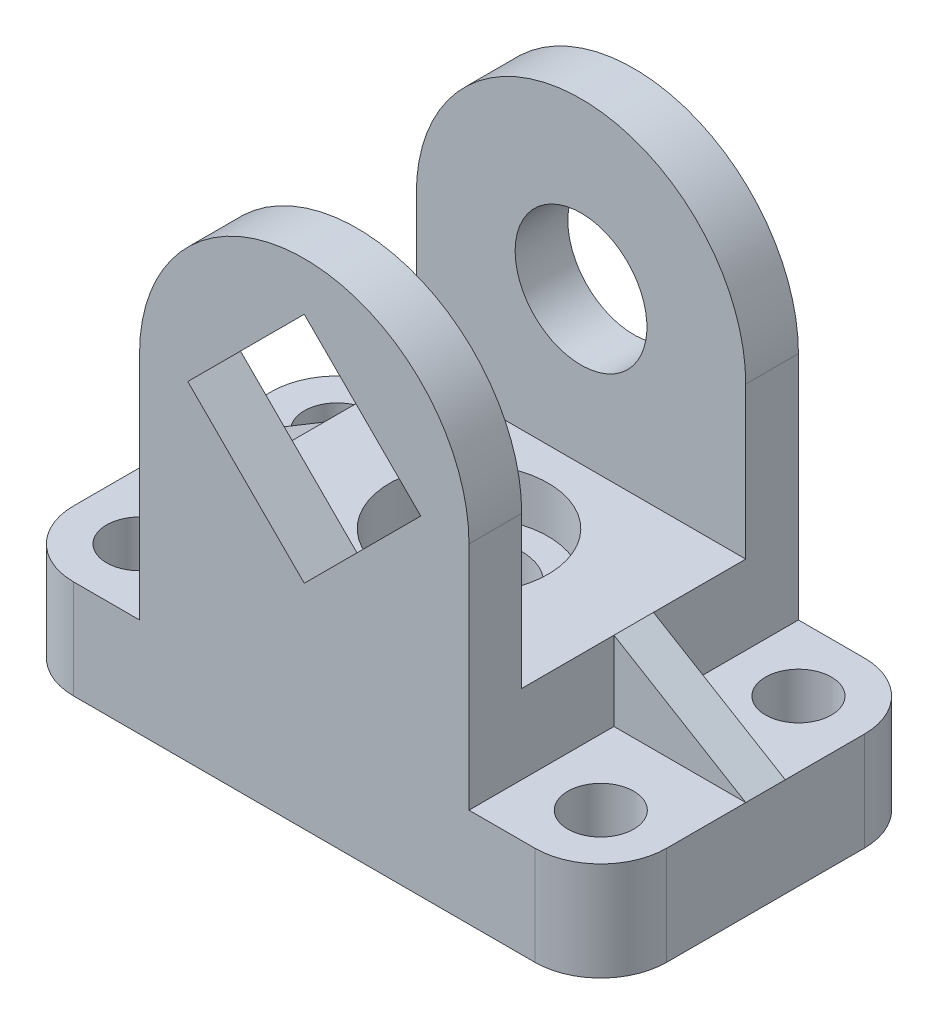
ISO-10303-21;
HEADER;
FILE_DESCRIPTION(('STEP AP214'),'2;1');
FILE_NAME('part.step','',(''),(''),'','','');
FILE_SCHEMA(('AUTOMOTIVE_DESIGN { 1 0 10303 214 1 1 1 1 }'));
ENDSEC;
DATA;
#1=APPLICATION_CONTEXT('core data for automotive mechanical design processes');
#2=APPLICATION_PROTOCOL_DEFINITION('international standard','automotive_design',2000,#1);
#3=PRODUCT_CONTEXT('',#1,'mechanical');
#4=PRODUCT('Part','Part','',(#3));
#5=PRODUCT_RELATED_PRODUCT_CATEGORY('part','',(#4));
#6=PRODUCT_DEFINITION_FORMATION('','',#4);
#7=PRODUCT_DEFINITION_CONTEXT('part definition',#1,'design');
#8=PRODUCT_DEFINITION('design','',#6,#7);
#9=PRODUCT_DEFINITION_SHAPE('','',#8);
#10=(LENGTH_UNIT() NAMED_UNIT(*) SI_UNIT(.MILLI.,.METRE.));
#11=(NAMED_UNIT(*) PLANE_ANGLE_UNIT() SI_UNIT($,.RADIAN.));
#12=(NAMED_UNIT(*) SI_UNIT($,.STERADIAN.) SOLID_ANGLE_UNIT());
#13=UNCERTAINTY_MEASURE_WITH_UNIT(LENGTH_MEASURE(1.E-05),#10,'distance_accuracy_value','');
#14=(GEOMETRIC_REPRESENTATION_CONTEXT(3) GLOBAL_UNCERTAINTY_ASSIGNED_CONTEXT((#13)) GLOBAL_UNIT_ASSIGNED_CONTEXT((#10,
#11,#12)) REPRESENTATION_CONTEXT('',''));
#15=CARTESIAN_POINT('',(0.,0.,0.));
#16=DIRECTION('',(0.,0.,1.));
#17=DIRECTION('',(1.,0.,0.));
#18=AXIS2_PLACEMENT_3D('',#15,#16,#17);
#19=CARTESIAN_POINT('',(-35.,15.,15.));
#20=DIRECTION('',(0.,-1.,0.));
#21=DIRECTION('',(0.,0.,-1.));
#22=AXIS2_PLACEMENT_3D('',#19,#20,#21);
#23=PLANE('',#22);
#24=CARTESIAN_POINT('',(-35.,15.,-15.));
#25=DIRECTION('',(0.,1.,0.));
#26=DIRECTION('',(0.,0.,1.));
#27=AXIS2_PLACEMENT_3D('',#24,#25,#26);
#28=CIRCLE('',#27,5.);
#29=CARTESIAN_POINT('',(-35.,15.,-10.));
#30=VERTEX_POINT('',#29);
#31=EDGE_CURVE('E380',#30,#30,#28,.T.);
#32=ORIENTED_EDGE('',*,*,#31,.F.);
#33=EDGE_LOOP('',(#32));
#34=FACE_BOUND('',#33,.T.);
#35=DIRECTION('',(-1.,0.,0.));
#36=VECTOR('',#35,1.);
#37=CARTESIAN_POINT('',(-35.,15.,-3.));
#38=LINE('',#37,#36);
#39=CARTESIAN_POINT('',(-25.,15.,-3.));
#40=VERTEX_POINT('',#39);
#41=CARTESIAN_POINT('',(-45.,15.,-3.));
#42=VERTEX_POINT('',#41);
#43=EDGE_CURVE('E230',#40,#42,#38,.T.);
#44=ORIENTED_EDGE('',*,*,#43,.F.);
#45=DIRECTION('',(0.,0.,1.));
#46=VECTOR('',#45,1.);
#47=CARTESIAN_POINT('',(-25.,15.,17.));
#48=LINE('',#47,#46);
#49=CARTESIAN_POINT('',(-25.,15.,-25.));
#50=VERTEX_POINT('',#49);
#51=EDGE_CURVE('E234',#50,#40,#48,.T.);
#52=ORIENTED_EDGE('',*,*,#51,.F.);
#53=DIRECTION('',(-1.,0.,0.));
#54=VECTOR('',#53,1.);
#55=CARTESIAN_POINT('',(-35.,15.,-25.));
#56=LINE('',#55,#54);
#57=CARTESIAN_POINT('',(-35.,15.,-25.));
#58=VERTEX_POINT('',#57);
#59=EDGE_CURVE('E396',#50,#58,#56,.T.);
#60=ORIENTED_EDGE('',*,*,#59,.T.);
#61=CARTESIAN_POINT('',(-35.,15.,-15.));
#62=DIRECTION('',(0.,1.,0.));
#63=DIRECTION('',(0.,0.,-1.));
#64=AXIS2_PLACEMENT_3D('',#61,#62,#63);
#65=CIRCLE('',#64,10.);
#66=CARTESIAN_POINT('',(-45.,15.,-15.));
#67=VERTEX_POINT('',#66);
#68=EDGE_CURVE('E399',#58,#67,#65,.T.);
#69=ORIENTED_EDGE('',*,*,#68,.T.);
#70=DIRECTION('',(0.,0.,1.));
#71=VECTOR('',#70,1.);
#72=CARTESIAN_POINT('',(-45.,15.,15.));
#73=LINE('',#72,#71);
#74=EDGE_CURVE('E401',#67,#42,#73,.T.);
#75=ORIENTED_EDGE('',*,*,#74,.T.);
#76=EDGE_LOOP('',(#44,#52,#60,#69,#75));
#77=FACE_BOUND('',#76,.T.);
#78=ADVANCED_FACE('F39',(#34,#77),#23,.F.);
#79=CARTESIAN_POINT('',(-25.,15.,17.));
#80=DIRECTION('',(-1.,0.,0.));
#81=DIRECTION('',(0.,0.,1.));
#82=AXIS2_PLACEMENT_3D('',#79,#80,#81);
#83=PLANE('',#82);
#84=ORIENTED_EDGE('',*,*,#51,.T.);
#85=DIRECTION('',(0.,1.,0.));
#86=VECTOR('',#85,1.);
#87=CARTESIAN_POINT('',(-25.,15.,-3.));
#88=LINE('',#87,#86);
#89=CARTESIAN_POINT('',(-25.,27.,-3.));
#90=VERTEX_POINT('',#89);
#91=EDGE_CURVE('E223',#40,#90,#88,.T.);
#92=ORIENTED_EDGE('',*,*,#91,.T.);
#93=DIRECTION('',(0.,0.,1.));
#94=VECTOR('',#93,1.);
#95=CARTESIAN_POINT('',(-25.,27.,-17.));
#96=LINE('',#95,#94);
#97=CARTESIAN_POINT('',(-25.,27.,-17.));
#98=VERTEX_POINT('',#97);
#99=EDGE_CURVE('E218',#98,#90,#96,.T.);
#100=ORIENTED_EDGE('',*,*,#99,.F.);
#101=DIRECTION('',(0.,-1.,0.));
#102=VECTOR('',#101,1.);
#103=CARTESIAN_POINT('',(-25.,15.,-17.));
#104=LINE('',#103,#102);
#105=CARTESIAN_POINT('',(-25.,50.,-17.));
#106=VERTEX_POINT('',#105);
#107=EDGE_CURVE('E497',#106,#98,#104,.T.);
#108=ORIENTED_EDGE('',*,*,#107,.F.);
#109=DIRECTION('',(0.,0.,-1.));
#110=VECTOR('',#109,1.);
#111=CARTESIAN_POINT('',(-25.,50.,-17.));
#112=LINE('',#111,#110);
#113=CARTESIAN_POINT('',(-25.,50.,-25.));
#114=VERTEX_POINT('',#113);
#115=EDGE_CURVE('E477',#106,#114,#112,.T.);
#116=ORIENTED_EDGE('',*,*,#115,.T.);
#117=DIRECTION('',(0.,-1.,0.));
#118=VECTOR('',#117,1.);
#119=CARTESIAN_POINT('',(-25.,15.,-25.));
#120=LINE('',#119,#118);
#121=EDGE_CURVE('E496',#114,#50,#120,.T.);
#122=ORIENTED_EDGE('',*,*,#121,.T.);
#123=EDGE_LOOP('',(#84,#92,#100,#108,#116,#122));
#124=FACE_BOUND('',#123,.T.);
#125=ADVANCED_FACE('F235',(#124),#83,.T.);
#126=CARTESIAN_POINT('',(35.,15.,-15.));
#127=DIRECTION('',(0.,1.,0.));
#128=DIRECTION('',(0.,0.,1.));
#129=AXIS2_PLACEMENT_3D('',#126,#127,#128);
#130=CIRCLE('',#129,5.);
#131=CARTESIAN_POINT('',(35.,15.,-10.));
#132=VERTEX_POINT('',#131);
#133=EDGE_CURVE('E371',#132,#132,#130,.T.);
#134=ORIENTED_EDGE('',*,*,#133,.F.);
#135=EDGE_LOOP('',(#134));
#136=FACE_BOUND('',#135,.T.);
#137=DIRECTION('',(-1.,0.,0.));
#138=VECTOR('',#137,1.);
#139=CARTESIAN_POINT('',(-35.,15.,-3.));
#140=LINE('',#139,#138);
#141=CARTESIAN_POINT('',(45.,15.,-3.));
#142=VERTEX_POINT('',#141);
#143=CARTESIAN_POINT('',(25.,15.,-3.));
#144=VERTEX_POINT('',#143);
#145=EDGE_CURVE('E256',#142,#144,#140,.T.);
#146=ORIENTED_EDGE('',*,*,#145,.F.);
#147=DIRECTION('',(0.,0.,-1.));
#148=VECTOR('',#147,1.);
#149=CARTESIAN_POINT('',(45.,15.,15.));
#150=LINE('',#149,#148);
#151=CARTESIAN_POINT('',(45.,15.,-15.));
#152=VERTEX_POINT('',#151);
#153=EDGE_CURVE('E388',#142,#152,#150,.T.);
#154=ORIENTED_EDGE('',*,*,#153,.T.);
#155=CARTESIAN_POINT('',(35.,15.,-15.));
#156=DIRECTION('',(0.,1.,0.));
#157=DIRECTION('',(0.,0.,-1.));
#158=AXIS2_PLACEMENT_3D('',#155,#156,#157);
#159=CIRCLE('',#158,10.);
#160=CARTESIAN_POINT('',(35.,15.,-25.));
#161=VERTEX_POINT('',#160);
#162=EDGE_CURVE('E392',#152,#161,#159,.T.);
#163=ORIENTED_EDGE('',*,*,#162,.T.);
#164=CARTESIAN_POINT('',(25.,15.,-25.));
#165=VERTEX_POINT('',#164);
#166=EDGE_CURVE('E400',#161,#165,#56,.T.);
#167=ORIENTED_EDGE('',*,*,#166,.T.);
#168=DIRECTION('',(0.,0.,1.));
#169=VECTOR('',#168,1.);
#170=CARTESIAN_POINT('',(25.,15.,17.));
#171=LINE('',#170,#169);
#172=EDGE_CURVE('E360',#165,#144,#171,.T.);
#173=ORIENTED_EDGE('',*,*,#172,.T.);
#174=EDGE_LOOP('',(#146,#154,#163,#167,#173));
#175=FACE_BOUND('',#174,.T.);
#176=ADVANCED_FACE('F304',(#136,#175),#23,.F.);
#177=CARTESIAN_POINT('',(25.,50.,17.));
#178=DIRECTION('',(1.,0.,0.));
#179=DIRECTION('',(0.,1.,0.));
#180=AXIS2_PLACEMENT_3D('',#177,#178,#179);
#181=PLANE('',#180);
#182=DIRECTION('',(0.,0.,-1.));
#183=VECTOR('',#182,1.);
#184=CARTESIAN_POINT('',(25.,27.,-17.));
#185=LINE('',#184,#183);
#186=CARTESIAN_POINT('',(25.,27.,-3.));
#187=VERTEX_POINT('',#186);
#188=CARTESIAN_POINT('',(25.,27.,-17.));
#189=VERTEX_POINT('',#188);
#190=EDGE_CURVE('E242',#187,#189,#185,.T.);
#191=ORIENTED_EDGE('',*,*,#190,.F.);
#192=DIRECTION('',(0.,-1.,0.));
#193=VECTOR('',#192,1.);
#194=CARTESIAN_POINT('',(25.,50.,-3.));
#195=LINE('',#194,#193);
#196=EDGE_CURVE('E257',#187,#144,#195,.T.);
#197=ORIENTED_EDGE('',*,*,#196,.T.);
#198=ORIENTED_EDGE('',*,*,#172,.F.);
#199=DIRECTION('',(0.,1.,0.));
#200=VECTOR('',#199,1.);
#201=CARTESIAN_POINT('',(25.,50.,-25.));
#202=LINE('',#201,#200);
#203=CARTESIAN_POINT('',(25.,50.,-25.));
#204=VERTEX_POINT('',#203);
#205=EDGE_CURVE('E493',#165,#204,#202,.T.);
#206=ORIENTED_EDGE('',*,*,#205,.T.);
#207=DIRECTION('',(0.,0.,-1.));
#208=VECTOR('',#207,1.);
#209=CARTESIAN_POINT('',(25.,50.,-17.));
#210=LINE('',#209,#208);
#211=CARTESIAN_POINT('',(25.,50.,-17.));
#212=VERTEX_POINT('',#211);
#213=EDGE_CURVE('E480',#212,#204,#210,.T.);
#214=ORIENTED_EDGE('',*,*,#213,.F.);
#215=DIRECTION('',(0.,1.,0.));
#216=VECTOR('',#215,1.);
#217=CARTESIAN_POINT('',(25.,50.,-17.));
#218=LINE('',#217,#216);
#219=EDGE_CURVE('E495',#189,#212,#218,.T.);
#220=ORIENTED_EDGE('',*,*,#219,.F.);
#221=EDGE_LOOP('',(#191,#197,#198,#206,#214,#220));
#222=FACE_BOUND('',#221,.T.);
#223=ADVANCED_FACE('F318',(#222),#181,.T.);
#224=CARTESIAN_POINT('',(-35.,15.,15.));
#225=DIRECTION('',(0.,1.,0.));
#226=DIRECTION('',(0.,0.,1.));
#227=AXIS2_PLACEMENT_3D('',#224,#225,#226);
#228=CIRCLE('',#227,5.);
#229=CARTESIAN_POINT('',(-35.,15.,20.));
#230=VERTEX_POINT('',#229);
#231=EDGE_CURVE('E338',#230,#230,#228,.T.);
#232=ORIENTED_EDGE('',*,*,#231,.F.);
#233=EDGE_LOOP('',(#232));
#234=FACE_BOUND('',#233,.T.);
#235=CARTESIAN_POINT('',(-25.,15.,3.));
#236=VERTEX_POINT('',#235);
#237=CARTESIAN_POINT('',(-25.,15.,25.));
#238=VERTEX_POINT('',#237);
#239=EDGE_CURVE('E337',#236,#238,#48,.T.);
#240=ORIENTED_EDGE('',*,*,#239,.F.);
#241=DIRECTION('',(-1.,0.,0.));
#242=VECTOR('',#241,1.);
#243=CARTESIAN_POINT('',(-35.,15.,3.));
#244=LINE('',#243,#242);
#245=CARTESIAN_POINT('',(-45.,15.,3.));
#246=VERTEX_POINT('',#245);
#247=EDGE_CURVE('E268',#236,#246,#244,.T.);
#248=ORIENTED_EDGE('',*,*,#247,.T.);
#249=CARTESIAN_POINT('',(-45.,15.,15.));
#250=VERTEX_POINT('',#249);
#251=EDGE_CURVE('E405',#246,#250,#73,.T.);
#252=ORIENTED_EDGE('',*,*,#251,.T.);
#253=CARTESIAN_POINT('',(-35.,15.,15.));
#254=DIRECTION('',(0.,1.,0.));
#255=DIRECTION('',(0.,0.,-1.));
#256=AXIS2_PLACEMENT_3D('',#253,#254,#255);
#257=CIRCLE('',#256,10.);
#258=CARTESIAN_POINT('',(-35.,15.,25.));
#259=VERTEX_POINT('',#258);
#260=EDGE_CURVE('E382',#250,#259,#257,.T.);
#261=ORIENTED_EDGE('',*,*,#260,.T.);
#262=DIRECTION('',(1.,0.,0.));
#263=VECTOR('',#262,1.);
#264=CARTESIAN_POINT('',(-35.,15.,25.));
#265=LINE('',#264,#263);
#266=EDGE_CURVE('E345',#259,#238,#265,.T.);
#267=ORIENTED_EDGE('',*,*,#266,.T.);
#268=EDGE_LOOP('',(#240,#248,#252,#261,#267));
#269=FACE_BOUND('',#268,.T.);
#270=ADVANCED_FACE('F308',(#234,#269),#23,.F.);
#271=CARTESIAN_POINT('',(35.,15.,15.));
#272=DIRECTION('',(0.,1.,0.));
#273=DIRECTION('',(0.,0.,1.));
#274=AXIS2_PLACEMENT_3D('',#271,#272,#273);
#275=CIRCLE('',#274,5.);
#276=CARTESIAN_POINT('',(35.,15.,20.));
#277=VERTEX_POINT('',#276);
#278=EDGE_CURVE('E363',#277,#277,#275,.T.);
#279=ORIENTED_EDGE('',*,*,#278,.F.);
#280=EDGE_LOOP('',(#279));
#281=FACE_BOUND('',#280,.T.);
#282=CARTESIAN_POINT('',(45.,15.,15.));
#283=VERTEX_POINT('',#282);
#284=CARTESIAN_POINT('',(45.,15.,3.));
#285=VERTEX_POINT('',#284);
#286=EDGE_CURVE('E393',#283,#285,#150,.T.);
#287=ORIENTED_EDGE('',*,*,#286,.T.);
#288=DIRECTION('',(-1.,0.,0.));
#289=VECTOR('',#288,1.);
#290=CARTESIAN_POINT('',(-35.,15.,3.));
#291=LINE('',#290,#289);
#292=CARTESIAN_POINT('',(25.,15.,3.));
#293=VERTEX_POINT('',#292);
#294=EDGE_CURVE('E249',#285,#293,#291,.T.);
#295=ORIENTED_EDGE('',*,*,#294,.T.);
#296=CARTESIAN_POINT('',(25.,15.,25.));
#297=VERTEX_POINT('',#296);
#298=EDGE_CURVE('E359',#293,#297,#171,.T.);
#299=ORIENTED_EDGE('',*,*,#298,.T.);
#300=CARTESIAN_POINT('',(35.,15.,25.));
#301=VERTEX_POINT('',#300);
#302=EDGE_CURVE('E384',#297,#301,#265,.T.);
#303=ORIENTED_EDGE('',*,*,#302,.T.);
#304=CARTESIAN_POINT('',(35.,15.,15.));
#305=DIRECTION('',(0.,1.,0.));
#306=DIRECTION('',(0.,0.,1.));
#307=AXIS2_PLACEMENT_3D('',#304,#305,#306);
#308=CIRCLE('',#307,10.);
#309=EDGE_CURVE('E389',#301,#283,#308,.T.);
#310=ORIENTED_EDGE('',*,*,#309,.T.);
#311=EDGE_LOOP('',(#287,#295,#299,#303,#310));
#312=FACE_BOUND('',#311,.T.);
#313=ADVANCED_FACE('F319',(#281,#312),#23,.F.);
#314=CARTESIAN_POINT('',(-35.,0.,15.));
#315=DIRECTION('',(0.,-1.,0.));
#316=DIRECTION('',(0.,0.,-1.));
#317=AXIS2_PLACEMENT_3D('',#314,#315,#316);
#318=PLANE('',#317);
#319=CARTESIAN_POINT('',(0.,0.,0.));
#320=DIRECTION('',(0.,-1.,0.));
#321=DIRECTION('',(0.,0.,-1.));
#322=AXIS2_PLACEMENT_3D('',#319,#320,#321);
#323=CIRCLE('',#322,8.00000000000001);
#324=CARTESIAN_POINT('',(0.,0.,-8.00000000000001));
#325=VERTEX_POINT('',#324);
#326=EDGE_CURVE('E43',#325,#325,#323,.T.);
#327=ORIENTED_EDGE('',*,*,#326,.F.);
#328=EDGE_LOOP('',(#327));
#329=FACE_BOUND('',#328,.T.);
#330=CARTESIAN_POINT('',(-35.,0.,15.));
#331=DIRECTION('',(0.,1.,0.));
#332=DIRECTION('',(0.,0.,-1.));
#333=AXIS2_PLACEMENT_3D('',#330,#331,#332);
#334=CIRCLE('',#333,10.);
#335=CARTESIAN_POINT('',(-45.,0.,15.));
#336=VERTEX_POINT('',#335);
#337=CARTESIAN_POINT('',(-35.,0.,25.));
#338=VERTEX_POINT('',#337);
#339=EDGE_CURVE('E379',#336,#338,#334,.T.);
#340=ORIENTED_EDGE('',*,*,#339,.F.);
#341=DIRECTION('',(0.,0.,1.));
#342=VECTOR('',#341,1.);
#343=CARTESIAN_POINT('',(-45.,0.,15.));
#344=LINE('',#343,#342);
#345=CARTESIAN_POINT('',(-45.,0.,-15.));
#346=VERTEX_POINT('',#345);
#347=EDGE_CURVE('E387',#346,#336,#344,.T.);
#348=ORIENTED_EDGE('',*,*,#347,.F.);
#349=CARTESIAN_POINT('',(-35.,0.,-15.));
#350=DIRECTION('',(0.,1.,0.));
#351=DIRECTION('',(0.,0.,-1.));
#352=AXIS2_PLACEMENT_3D('',#349,#350,#351);
#353=CIRCLE('',#352,10.);
#354=CARTESIAN_POINT('',(-35.,0.,-25.));
#355=VERTEX_POINT('',#354);
#356=EDGE_CURVE('E420',#355,#346,#353,.T.);
#357=ORIENTED_EDGE('',*,*,#356,.F.);
#358=DIRECTION('',(-1.,0.,0.));
#359=VECTOR('',#358,1.);
#360=CARTESIAN_POINT('',(-35.,0.,-25.));
#361=LINE('',#360,#359);
#362=CARTESIAN_POINT('',(35.,0.,-25.));
#363=VERTEX_POINT('',#362);
#364=EDGE_CURVE('E417',#363,#355,#361,.T.);
#365=ORIENTED_EDGE('',*,*,#364,.F.);
#366=CARTESIAN_POINT('',(35.,0.,-15.));
#367=DIRECTION('',(0.,1.,0.));
#368=DIRECTION('',(0.,0.,-1.));
#369=AXIS2_PLACEMENT_3D('',#366,#367,#368);
#370=CIRCLE('',#369,10.);
#371=CARTESIAN_POINT('',(45.,0.,-15.));
#372=VERTEX_POINT('',#371);
#373=EDGE_CURVE('E414',#372,#363,#370,.T.);
#374=ORIENTED_EDGE('',*,*,#373,.F.);
#375=DIRECTION('',(0.,0.,-1.));
#376=VECTOR('',#375,1.);
#377=CARTESIAN_POINT('',(45.,0.,15.));
#378=LINE('',#377,#376);
#379=CARTESIAN_POINT('',(45.,0.,15.));
#380=VERTEX_POINT('',#379);
#381=EDGE_CURVE('E412',#380,#372,#378,.T.);
#382=ORIENTED_EDGE('',*,*,#381,.F.);
#383=CARTESIAN_POINT('',(35.,0.,15.));
#384=DIRECTION('',(0.,1.,0.));
#385=DIRECTION('',(0.,0.,1.));
#386=AXIS2_PLACEMENT_3D('',#383,#384,#385);
#387=CIRCLE('',#386,10.);
#388=CARTESIAN_POINT('',(35.,0.,25.));
#389=VERTEX_POINT('',#388);
#390=EDGE_CURVE('E411',#389,#380,#387,.T.);
#391=ORIENTED_EDGE('',*,*,#390,.F.);
#392=DIRECTION('',(1.,0.,0.));
#393=VECTOR('',#392,1.);
#394=CARTESIAN_POINT('',(-35.,0.,25.));
#395=LINE('',#394,#393);
#396=EDGE_CURVE('E407',#338,#389,#395,.T.);
#397=ORIENTED_EDGE('',*,*,#396,.F.);
#398=EDGE_LOOP('',(#340,#348,#357,#365,#374,#382,#391,#397));
#399=FACE_BOUND('',#398,.T.);
#400=CARTESIAN_POINT('',(-35.,0.,15.));
#401=DIRECTION('',(0.,1.,0.));
#402=DIRECTION('',(0.,0.,1.));
#403=AXIS2_PLACEMENT_3D('',#400,#401,#402);
#404=CIRCLE('',#403,5.);
#405=CARTESIAN_POINT('',(-35.,0.,20.));
#406=VERTEX_POINT('',#405);
#407=EDGE_CURVE('E365',#406,#406,#404,.T.);
#408=ORIENTED_EDGE('',*,*,#407,.T.);
#409=EDGE_LOOP('',(#408));
#410=FACE_BOUND('',#409,.T.);
#411=CARTESIAN_POINT('',(35.,0.,15.));
#412=DIRECTION('',(0.,1.,0.));
#413=DIRECTION('',(0.,0.,1.));
#414=AXIS2_PLACEMENT_3D('',#411,#412,#413);
#415=CIRCLE('',#414,5.);
#416=CARTESIAN_POINT('',(35.,0.,20.));
#417=VERTEX_POINT('',#416);
#418=EDGE_CURVE('E349',#417,#417,#415,.T.);
#419=ORIENTED_EDGE('',*,*,#418,.T.);
#420=EDGE_LOOP('',(#419));
#421=FACE_BOUND('',#420,.T.);
#422=CARTESIAN_POINT('',(-35.,0.,-15.));
#423=DIRECTION('',(0.,1.,0.));
#424=DIRECTION('',(0.,0.,1.));
#425=AXIS2_PLACEMENT_3D('',#422,#423,#424);
#426=CIRCLE('',#425,5.);
#427=CARTESIAN_POINT('',(-35.,0.,-10.));
#428=VERTEX_POINT('',#427);
#429=EDGE_CURVE('E372',#428,#428,#426,.T.);
#430=ORIENTED_EDGE('',*,*,#429,.T.);
#431=EDGE_LOOP('',(#430));
#432=FACE_BOUND('',#431,.T.);
#433=CARTESIAN_POINT('',(35.,0.,-15.));
#434=DIRECTION('',(0.,1.,0.));
#435=DIRECTION('',(0.,0.,1.));
#436=AXIS2_PLACEMENT_3D('',#433,#434,#435);
#437=CIRCLE('',#436,5.);
#438=CARTESIAN_POINT('',(35.,0.,-10.));
#439=VERTEX_POINT('',#438);
#440=EDGE_CURVE('E366',#439,#439,#437,.T.);
#441=ORIENTED_EDGE('',*,*,#440,.T.);
#442=EDGE_LOOP('',(#441));
#443=FACE_BOUND('',#442,.T.);
#444=ADVANCED_FACE('F330',(#329,#399,#410,#421,#432,#443),#318,.T.);
#445=CARTESIAN_POINT('',(-35.,15.,15.));
#446=DIRECTION('',(0.,-1.,0.));
#447=DIRECTION('',(0.,0.,-1.));
#448=AXIS2_PLACEMENT_3D('',#445,#446,#447);
#449=CYLINDRICAL_SURFACE('',#448,10.);
#450=ORIENTED_EDGE('',*,*,#339,.T.);
#451=DIRECTION('',(0.,-1.,0.));
#452=VECTOR('',#451,1.);
#453=CARTESIAN_POINT('',(-35.,15.,25.));
#454=LINE('',#453,#452);
#455=EDGE_CURVE('E11',#259,#338,#454,.T.);
#456=ORIENTED_EDGE('',*,*,#455,.F.);
#457=ORIENTED_EDGE('',*,*,#260,.F.);
#458=DIRECTION('',(0.,-1.,0.));
#459=VECTOR('',#458,1.);
#460=CARTESIAN_POINT('',(-45.,15.,15.));
#461=LINE('',#460,#459);
#462=EDGE_CURVE('E408',#250,#336,#461,.T.);
#463=ORIENTED_EDGE('',*,*,#462,.T.);
#464=EDGE_LOOP('',(#450,#456,#457,#463));
#465=FACE_BOUND('',#464,.T.);
#466=ADVANCED_FACE('F41',(#465),#449,.T.);
#467=CARTESIAN_POINT('',(-35.,15.,25.));
#468=DIRECTION('',(0.,0.,-1.));
#469=DIRECTION('',(-1.,0.,0.));
#470=AXIS2_PLACEMENT_3D('',#467,#468,#469);
#471=PLANE('',#470);
#472=DIRECTION('',(0.707106781186547,0.707106781186548,0.));
#473=VECTOR('',#472,1.);
#474=CARTESIAN_POINT('',(17.6776695296637,50.,25.));
#475=LINE('',#474,#473);
#476=CARTESIAN_POINT('',(0.,32.3223304703363,25.));
#477=VERTEX_POINT('',#476);
#478=CARTESIAN_POINT('',(17.6776695296637,50.,25.));
#479=VERTEX_POINT('',#478);
#480=EDGE_CURVE('E525',#477,#479,#475,.T.);
#481=ORIENTED_EDGE('',*,*,#480,.F.);
#482=DIRECTION('',(0.707106781186547,-0.707106781186548,0.));
#483=VECTOR('',#482,1.);
#484=CARTESIAN_POINT('',(0.,32.3223304703363,25.));
#485=LINE('',#484,#483);
#486=CARTESIAN_POINT('',(-17.6776695296637,50.,25.));
#487=VERTEX_POINT('',#486);
#488=EDGE_CURVE('E524',#487,#477,#485,.T.);
#489=ORIENTED_EDGE('',*,*,#488,.F.);
#490=DIRECTION('',(-0.707106781186547,-0.707106781186548,0.));
#491=VECTOR('',#490,1.);
#492=CARTESIAN_POINT('',(-17.6776695296637,50.,25.));
#493=LINE('',#492,#491);
#494=CARTESIAN_POINT('',(0.,67.6776695296637,25.));
#495=VERTEX_POINT('',#494);
#496=EDGE_CURVE('E513',#495,#487,#493,.T.);
#497=ORIENTED_EDGE('',*,*,#496,.F.);
#498=DIRECTION('',(-0.707106781186548,0.707106781186547,0.));
#499=VECTOR('',#498,1.);
#500=CARTESIAN_POINT('',(0.,67.6776695296637,25.));
#501=LINE('',#500,#499);
#502=EDGE_CURVE('E517',#479,#495,#501,.T.);
#503=ORIENTED_EDGE('',*,*,#502,.F.);
#504=EDGE_LOOP('',(#481,#489,#497,#503));
#505=FACE_BOUND('',#504,.T.);
#506=ORIENTED_EDGE('',*,*,#396,.T.);
#507=DIRECTION('',(0.,-1.,0.));
#508=VECTOR('',#507,1.);
#509=CARTESIAN_POINT('',(35.,15.,25.));
#510=LINE('',#509,#508);
#511=EDGE_CURVE('E48',#301,#389,#510,.T.);
#512=ORIENTED_EDGE('',*,*,#511,.F.);
#513=ORIENTED_EDGE('',*,*,#302,.F.);
#514=DIRECTION('',(0.,1.,0.));
#515=VECTOR('',#514,1.);
#516=CARTESIAN_POINT('',(25.,50.,25.));
#517=LINE('',#516,#515);
#518=CARTESIAN_POINT('',(25.,50.,25.));
#519=VERTEX_POINT('',#518);
#520=EDGE_CURVE('E471',#297,#519,#517,.T.);
#521=ORIENTED_EDGE('',*,*,#520,.T.);
#522=CARTESIAN_POINT('',(0.,50.,25.));
#523=DIRECTION('',(0.,0.,1.));
#524=DIRECTION('',(-1.,0.,0.));
#525=AXIS2_PLACEMENT_3D('',#522,#523,#524);
#526=CIRCLE('',#525,25.);
#527=CARTESIAN_POINT('',(-25.,50.,25.));
#528=VERTEX_POINT('',#527);
#529=EDGE_CURVE('E474',#519,#528,#526,.T.);
#530=ORIENTED_EDGE('',*,*,#529,.T.);
#531=DIRECTION('',(0.,-1.,0.));
#532=VECTOR('',#531,1.);
#533=CARTESIAN_POINT('',(-25.,15.,25.));
#534=LINE('',#533,#532);
#535=EDGE_CURVE('E351',#528,#238,#534,.T.);
#536=ORIENTED_EDGE('',*,*,#535,.T.);
#537=ORIENTED_EDGE('',*,*,#266,.F.);
#538=ORIENTED_EDGE('',*,*,#455,.T.);
#539=EDGE_LOOP('',(#506,#512,#513,#521,#530,#536,#537,#538));
#540=FACE_BOUND('',#539,.T.);
#541=ADVANCED_FACE('F473',(#505,#540),#471,.F.);
#542=CARTESIAN_POINT('',(35.,15.,15.));
#543=DIRECTION('',(0.,-1.,0.));
#544=DIRECTION('',(0.,0.,-1.));
#545=AXIS2_PLACEMENT_3D('',#542,#543,#544);
#546=CYLINDRICAL_SURFACE('',#545,10.);
#547=ORIENTED_EDGE('',*,*,#390,.T.);
#548=DIRECTION('',(0.,-1.,0.));
#549=VECTOR('',#548,1.);
#550=CARTESIAN_POINT('',(45.,15.,15.));
#551=LINE('',#550,#549);
#552=EDGE_CURVE('E436',#283,#380,#551,.T.);
#553=ORIENTED_EDGE('',*,*,#552,.F.);
#554=ORIENTED_EDGE('',*,*,#309,.F.);
#555=ORIENTED_EDGE('',*,*,#511,.T.);
#556=EDGE_LOOP('',(#547,#553,#554,#555));
#557=FACE_BOUND('',#556,.T.);
#558=ADVANCED_FACE('F441',(#557),#546,.T.);
#559=CARTESIAN_POINT('',(45.,15.,15.));
#560=DIRECTION('',(-1.,0.,0.));
#561=DIRECTION('',(0.,0.,1.));
#562=AXIS2_PLACEMENT_3D('',#559,#560,#561);
#563=PLANE('',#562);
#564=ORIENTED_EDGE('',*,*,#381,.T.);
#565=DIRECTION('',(0.,-1.,0.));
#566=VECTOR('',#565,1.);
#567=CARTESIAN_POINT('',(45.,15.,-15.));
#568=LINE('',#567,#566);
#569=EDGE_CURVE('E433',#152,#372,#568,.T.);
#570=ORIENTED_EDGE('',*,*,#569,.F.);
#571=ORIENTED_EDGE('',*,*,#153,.F.);
#572=DIRECTION('',(0.,0.,1.));
#573=VECTOR('',#572,1.);
#574=CARTESIAN_POINT('',(45.,15.,15.));
#575=LINE('',#574,#573);
#576=EDGE_CURVE('E250',#285,#142,#575,.F.);
#577=ORIENTED_EDGE('',*,*,#576,.F.);
#578=ORIENTED_EDGE('',*,*,#286,.F.);
#579=ORIENTED_EDGE('',*,*,#552,.T.);
#580=EDGE_LOOP('',(#564,#570,#571,#577,#578,#579));
#581=FACE_BOUND('',#580,.T.);
#582=ADVANCED_FACE('F457',(#581),#563,.F.);
#583=CARTESIAN_POINT('',(35.,15.,-15.));
#584=DIRECTION('',(0.,-1.,0.));
#585=DIRECTION('',(0.,0.,-1.));
#586=AXIS2_PLACEMENT_3D('',#583,#584,#585);
#587=CYLINDRICAL_SURFACE('',#586,10.);
#588=ORIENTED_EDGE('',*,*,#373,.T.);
#589=DIRECTION('',(0.,-1.,0.));
#590=VECTOR('',#589,1.);
#591=CARTESIAN_POINT('',(35.,15.,-25.));
#592=LINE('',#591,#590);
#593=EDGE_CURVE('E429',#161,#363,#592,.T.);
#594=ORIENTED_EDGE('',*,*,#593,.F.);
#595=ORIENTED_EDGE('',*,*,#162,.F.);
#596=ORIENTED_EDGE('',*,*,#569,.T.);
#597=EDGE_LOOP('',(#588,#594,#595,#596));
#598=FACE_BOUND('',#597,.T.);
#599=ADVANCED_FACE('F463',(#598),#587,.T.);
#600=CARTESIAN_POINT('',(-35.,15.,-25.));
#601=DIRECTION('',(0.,0.,1.));
#602=DIRECTION('',(1.,0.,0.));
#603=AXIS2_PLACEMENT_3D('',#600,#601,#602);
#604=PLANE('',#603);
#605=CARTESIAN_POINT('',(0.,50.,-25.));
#606=DIRECTION('',(0.,0.,-1.));
#607=DIRECTION('',(-1.,0.,0.));
#608=AXIS2_PLACEMENT_3D('',#605,#606,#607);
#609=CIRCLE('',#608,10.);
#610=CARTESIAN_POINT('',(-10.,50.,-25.));
#611=VERTEX_POINT('',#610);
#612=EDGE_CURVE('E538',#611,#611,#609,.T.);
#613=ORIENTED_EDGE('',*,*,#612,.F.);
#614=EDGE_LOOP('',(#613));
#615=FACE_BOUND('',#614,.T.);
#616=ORIENTED_EDGE('',*,*,#364,.T.);
#617=DIRECTION('',(0.,-1.,0.));
#618=VECTOR('',#617,1.);
#619=CARTESIAN_POINT('',(-35.,15.,-25.));
#620=LINE('',#619,#618);
#621=EDGE_CURVE('E430',#58,#355,#620,.T.);
#622=ORIENTED_EDGE('',*,*,#621,.F.);
#623=ORIENTED_EDGE('',*,*,#59,.F.);
#624=ORIENTED_EDGE('',*,*,#121,.F.);
#625=CARTESIAN_POINT('',(0.,50.,-25.));
#626=DIRECTION('',(0.,0.,1.));
#627=DIRECTION('',(-1.,0.,0.));
#628=AXIS2_PLACEMENT_3D('',#625,#626,#627);
#629=CIRCLE('',#628,25.);
#630=EDGE_CURVE('E500',#204,#114,#629,.T.);
#631=ORIENTED_EDGE('',*,*,#630,.F.);
#632=ORIENTED_EDGE('',*,*,#205,.F.);
#633=ORIENTED_EDGE('',*,*,#166,.F.);
#634=ORIENTED_EDGE('',*,*,#593,.T.);
#635=EDGE_LOOP('',(#616,#622,#623,#624,#631,#632,#633,#634));
#636=FACE_BOUND('',#635,.T.);
#637=ADVANCED_FACE('F565',(#615,#636),#604,.F.);
#638=CARTESIAN_POINT('',(-35.,15.,-15.));
#639=DIRECTION('',(0.,-1.,0.));
#640=DIRECTION('',(0.,0.,-1.));
#641=AXIS2_PLACEMENT_3D('',#638,#639,#640);
#642=CYLINDRICAL_SURFACE('',#641,10.);
#643=ORIENTED_EDGE('',*,*,#356,.T.);
#644=DIRECTION('',(0.,-1.,0.));
#645=VECTOR('',#644,1.);
#646=CARTESIAN_POINT('',(-45.,15.,-15.));
#647=LINE('',#646,#645);
#648=EDGE_CURVE('E424',#67,#346,#647,.T.);
#649=ORIENTED_EDGE('',*,*,#648,.F.);
#650=ORIENTED_EDGE('',*,*,#68,.F.);
#651=ORIENTED_EDGE('',*,*,#621,.T.);
#652=EDGE_LOOP('',(#643,#649,#650,#651));
#653=FACE_BOUND('',#652,.T.);
#654=ADVANCED_FACE('F822',(#653),#642,.T.);
#655=CARTESIAN_POINT('',(-45.,15.,15.));
#656=DIRECTION('',(1.,0.,0.));
#657=DIRECTION('',(0.,0.,-1.));
#658=AXIS2_PLACEMENT_3D('',#655,#656,#657);
#659=PLANE('',#658);
#660=ORIENTED_EDGE('',*,*,#251,.F.);
#661=DIRECTION('',(0.,0.,1.));
#662=VECTOR('',#661,1.);
#663=CARTESIAN_POINT('',(-45.,15.,15.));
#664=LINE('',#663,#662);
#665=EDGE_CURVE('E264',#42,#246,#664,.T.);
#666=ORIENTED_EDGE('',*,*,#665,.F.);
#667=ORIENTED_EDGE('',*,*,#74,.F.);
#668=ORIENTED_EDGE('',*,*,#648,.T.);
#669=ORIENTED_EDGE('',*,*,#347,.T.);
#670=ORIENTED_EDGE('',*,*,#462,.F.);
#671=EDGE_LOOP('',(#660,#666,#667,#668,#669,#670));
#672=FACE_BOUND('',#671,.T.);
#673=ADVANCED_FACE('F566',(#672),#659,.F.);
#674=CARTESIAN_POINT('',(-35.,15.,-15.));
#675=DIRECTION('',(0.,-1.,0.));
#676=DIRECTION('',(0.,0.,-1.));
#677=AXIS2_PLACEMENT_3D('',#674,#675,#676);
#678=CYLINDRICAL_SURFACE('',#677,5.);
#679=ORIENTED_EDGE('',*,*,#31,.T.);
#680=EDGE_LOOP('',(#679));
#681=FACE_BOUND('',#680,.T.);
#682=ORIENTED_EDGE('',*,*,#429,.F.);
#683=EDGE_LOOP('',(#682));
#684=FACE_BOUND('',#683,.T.);
#685=ADVANCED_FACE('F810',(#681,#684),#678,.F.);
#686=CARTESIAN_POINT('',(35.,15.,-15.));
#687=DIRECTION('',(0.,-1.,0.));
#688=DIRECTION('',(0.,0.,-1.));
#689=AXIS2_PLACEMENT_3D('',#686,#687,#688);
#690=CYLINDRICAL_SURFACE('',#689,5.);
#691=ORIENTED_EDGE('',*,*,#133,.T.);
#692=EDGE_LOOP('',(#691));
#693=FACE_BOUND('',#692,.T.);
#694=ORIENTED_EDGE('',*,*,#440,.F.);
#695=EDGE_LOOP('',(#694));
#696=FACE_BOUND('',#695,.T.);
#697=ADVANCED_FACE('F797',(#693,#696),#690,.F.);
#698=CARTESIAN_POINT('',(-35.,15.,15.));
#699=DIRECTION('',(0.,-1.,0.));
#700=DIRECTION('',(0.,0.,-1.));
#701=AXIS2_PLACEMENT_3D('',#698,#699,#700);
#702=CYLINDRICAL_SURFACE('',#701,5.);
#703=ORIENTED_EDGE('',*,*,#231,.T.);
#704=EDGE_LOOP('',(#703));
#705=FACE_BOUND('',#704,.T.);
#706=ORIENTED_EDGE('',*,*,#407,.F.);
#707=EDGE_LOOP('',(#706));
#708=FACE_BOUND('',#707,.T.);
#709=ADVANCED_FACE('F789',(#705,#708),#702,.F.);
#710=CARTESIAN_POINT('',(35.,15.,15.));
#711=DIRECTION('',(0.,-1.,0.));
#712=DIRECTION('',(0.,0.,-1.));
#713=AXIS2_PLACEMENT_3D('',#710,#711,#712);
#714=CYLINDRICAL_SURFACE('',#713,5.);
#715=ORIENTED_EDGE('',*,*,#278,.T.);
#716=EDGE_LOOP('',(#715));
#717=FACE_BOUND('',#716,.T.);
#718=ORIENTED_EDGE('',*,*,#418,.F.);
#719=EDGE_LOOP('',(#718));
#720=FACE_BOUND('',#719,.T.);
#721=ADVANCED_FACE('F779',(#717,#720),#714,.F.);
#722=DIRECTION('',(0.,1.,0.));
#723=VECTOR('',#722,1.);
#724=CARTESIAN_POINT('',(-25.,15.,3.));
#725=LINE('',#724,#723);
#726=CARTESIAN_POINT('',(-25.,27.,3.));
#727=VERTEX_POINT('',#726);
#728=EDGE_CURVE('E271',#236,#727,#725,.T.);
#729=ORIENTED_EDGE('',*,*,#728,.F.);
#730=ORIENTED_EDGE('',*,*,#239,.T.);
#731=ORIENTED_EDGE('',*,*,#535,.F.);
#732=DIRECTION('',(0.,0.,1.));
#733=VECTOR('',#732,1.);
#734=CARTESIAN_POINT('',(-25.,50.,17.));
#735=LINE('',#734,#733);
#736=CARTESIAN_POINT('',(-25.,50.,17.));
#737=VERTEX_POINT('',#736);
#738=EDGE_CURVE('E350',#737,#528,#735,.T.);
#739=ORIENTED_EDGE('',*,*,#738,.F.);
#740=DIRECTION('',(0.,-1.,0.));
#741=VECTOR('',#740,1.);
#742=CARTESIAN_POINT('',(-25.,15.,17.));
#743=LINE('',#742,#741);
#744=CARTESIAN_POINT('',(-25.,27.,17.));
#745=VERTEX_POINT('',#744);
#746=EDGE_CURVE('E483',#737,#745,#743,.T.);
#747=ORIENTED_EDGE('',*,*,#746,.T.);
#748=EDGE_CURVE('E219',#727,#745,#96,.T.);
#749=ORIENTED_EDGE('',*,*,#748,.F.);
#750=EDGE_LOOP('',(#729,#730,#731,#739,#747,#749));
#751=FACE_BOUND('',#750,.T.);
#752=ADVANCED_FACE('F315',(#751),#83,.T.);
#753=CARTESIAN_POINT('',(0.,50.,17.));
#754=DIRECTION('',(0.,0.,1.));
#755=DIRECTION('',(1.,0.,0.));
#756=AXIS2_PLACEMENT_3D('',#753,#754,#755);
#757=CYLINDRICAL_SURFACE('',#756,25.);
#758=ORIENTED_EDGE('',*,*,#529,.F.);
#759=DIRECTION('',(0.,0.,1.));
#760=VECTOR('',#759,1.);
#761=CARTESIAN_POINT('',(25.,50.,17.));
#762=LINE('',#761,#760);
#763=CARTESIAN_POINT('',(25.,50.,17.));
#764=VERTEX_POINT('',#763);
#765=EDGE_CURVE('E348',#764,#519,#762,.T.);
#766=ORIENTED_EDGE('',*,*,#765,.F.);
#767=CARTESIAN_POINT('',(0.,50.,17.));
#768=DIRECTION('',(0.,0.,1.));
#769=DIRECTION('',(-1.,0.,0.));
#770=AXIS2_PLACEMENT_3D('',#767,#768,#769);
#771=CIRCLE('',#770,25.);
#772=EDGE_CURVE('E486',#764,#737,#771,.T.);
#773=ORIENTED_EDGE('',*,*,#772,.T.);
#774=ORIENTED_EDGE('',*,*,#738,.T.);
#775=EDGE_LOOP('',(#758,#766,#773,#774));
#776=FACE_BOUND('',#775,.T.);
#777=ADVANCED_FACE('F766',(#776),#757,.T.);
#778=DIRECTION('',(0.,-1.,0.));
#779=VECTOR('',#778,1.);
#780=CARTESIAN_POINT('',(25.,50.,3.));
#781=LINE('',#780,#779);
#782=CARTESIAN_POINT('',(25.,27.,3.));
#783=VERTEX_POINT('',#782);
#784=EDGE_CURVE('E255',#783,#293,#781,.T.);
#785=ORIENTED_EDGE('',*,*,#784,.F.);
#786=CARTESIAN_POINT('',(25.,27.,17.));
#787=VERTEX_POINT('',#786);
#788=EDGE_CURVE('E542',#787,#783,#185,.T.);
#789=ORIENTED_EDGE('',*,*,#788,.F.);
#790=DIRECTION('',(0.,1.,0.));
#791=VECTOR('',#790,1.);
#792=CARTESIAN_POINT('',(25.,50.,17.));
#793=LINE('',#792,#791);
#794=EDGE_CURVE('E487',#787,#764,#793,.T.);
#795=ORIENTED_EDGE('',*,*,#794,.T.);
#796=ORIENTED_EDGE('',*,*,#765,.T.);
#797=ORIENTED_EDGE('',*,*,#520,.F.);
#798=ORIENTED_EDGE('',*,*,#298,.F.);
#799=EDGE_LOOP('',(#785,#789,#795,#796,#797,#798));
#800=FACE_BOUND('',#799,.T.);
#801=ADVANCED_FACE('F335',(#800),#181,.T.);
#802=CARTESIAN_POINT('',(0.,50.,17.));
#803=DIRECTION('',(0.,0.,-1.));
#804=DIRECTION('',(-1.,0.,0.));
#805=AXIS2_PLACEMENT_3D('',#802,#803,#804);
#806=PLANE('',#805);
#807=DIRECTION('',(1.,0.,0.));
#808=VECTOR('',#807,1.);
#809=CARTESIAN_POINT('',(-25.,27.,17.));
#810=LINE('',#809,#808);
#811=EDGE_CURVE('E245',#745,#787,#810,.T.);
#812=ORIENTED_EDGE('',*,*,#811,.F.);
#813=ORIENTED_EDGE('',*,*,#746,.F.);
#814=ORIENTED_EDGE('',*,*,#772,.F.);
#815=ORIENTED_EDGE('',*,*,#794,.F.);
#816=EDGE_LOOP('',(#812,#813,#814,#815));
#817=FACE_BOUND('',#816,.T.);
#818=DIRECTION('',(0.707106781186547,-0.707106781186548,0.));
#819=VECTOR('',#818,1.);
#820=CARTESIAN_POINT('',(0.,32.3223304703363,17.));
#821=LINE('',#820,#819);
#822=CARTESIAN_POINT('',(-17.6776695296637,50.,17.));
#823=VERTEX_POINT('',#822);
#824=CARTESIAN_POINT('',(0.,32.3223304703363,17.));
#825=VERTEX_POINT('',#824);
#826=EDGE_CURVE('E516',#823,#825,#821,.T.);
#827=ORIENTED_EDGE('',*,*,#826,.T.);
#828=DIRECTION('',(0.707106781186547,0.707106781186548,0.));
#829=VECTOR('',#828,1.);
#830=CARTESIAN_POINT('',(17.6776695296637,50.,17.));
#831=LINE('',#830,#829);
#832=CARTESIAN_POINT('',(17.6776695296637,50.,17.));
#833=VERTEX_POINT('',#832);
#834=EDGE_CURVE('E531',#825,#833,#831,.T.);
#835=ORIENTED_EDGE('',*,*,#834,.T.);
#836=DIRECTION('',(-0.707106781186548,0.707106781186547,0.));
#837=VECTOR('',#836,1.);
#838=CARTESIAN_POINT('',(0.,67.6776695296637,17.));
#839=LINE('',#838,#837);
#840=CARTESIAN_POINT('',(0.,67.6776695296637,17.));
#841=VERTEX_POINT('',#840);
#842=EDGE_CURVE('E529',#833,#841,#839,.T.);
#843=ORIENTED_EDGE('',*,*,#842,.T.);
#844=DIRECTION('',(-0.707106781186547,-0.707106781186548,0.));
#845=VECTOR('',#844,1.);
#846=CARTESIAN_POINT('',(-17.6776695296637,50.,17.));
#847=LINE('',#846,#845);
#848=EDGE_CURVE('E509',#841,#823,#847,.T.);
#849=ORIENTED_EDGE('',*,*,#848,.T.);
#850=EDGE_LOOP('',(#827,#835,#843,#849));
#851=FACE_BOUND('',#850,.T.);
#852=ADVANCED_FACE('F576',(#817,#851),#806,.T.);
#853=CARTESIAN_POINT('',(0.,50.,-17.));
#854=DIRECTION('',(0.,0.,-1.));
#855=DIRECTION('',(-1.,0.,0.));
#856=AXIS2_PLACEMENT_3D('',#853,#854,#855);
#857=CYLINDRICAL_SURFACE('',#856,25.);
#858=ORIENTED_EDGE('',*,*,#630,.T.);
#859=ORIENTED_EDGE('',*,*,#115,.F.);
#860=CARTESIAN_POINT('',(0.,50.,-17.));
#861=DIRECTION('',(0.,0.,1.));
#862=DIRECTION('',(-1.,0.,0.));
#863=AXIS2_PLACEMENT_3D('',#860,#861,#862);
#864=CIRCLE('',#863,25.);
#865=EDGE_CURVE('E501',#212,#106,#864,.T.);
#866=ORIENTED_EDGE('',*,*,#865,.F.);
#867=ORIENTED_EDGE('',*,*,#213,.T.);
#868=EDGE_LOOP('',(#858,#859,#866,#867));
#869=FACE_BOUND('',#868,.T.);
#870=ADVANCED_FACE('F556',(#869),#857,.T.);
#871=CARTESIAN_POINT('',(0.,50.,-17.));
#872=DIRECTION('',(0.,0.,1.));
#873=DIRECTION('',(-1.,0.,0.));
#874=AXIS2_PLACEMENT_3D('',#871,#872,#873);
#875=PLANE('',#874);
#876=DIRECTION('',(-1.,0.,0.));
#877=VECTOR('',#876,1.);
#878=CARTESIAN_POINT('',(-25.,27.,-17.));
#879=LINE('',#878,#877);
#880=EDGE_CURVE('E243',#189,#98,#879,.T.);
#881=ORIENTED_EDGE('',*,*,#880,.F.);
#882=ORIENTED_EDGE('',*,*,#219,.T.);
#883=ORIENTED_EDGE('',*,*,#865,.T.);
#884=ORIENTED_EDGE('',*,*,#107,.T.);
#885=EDGE_LOOP('',(#881,#882,#883,#884));
#886=FACE_BOUND('',#885,.T.);
#887=CARTESIAN_POINT('',(0.,50.,-17.));
#888=DIRECTION('',(0.,0.,-1.));
#889=DIRECTION('',(-1.,0.,0.));
#890=AXIS2_PLACEMENT_3D('',#887,#888,#889);
#891=CIRCLE('',#890,10.);
#892=CARTESIAN_POINT('',(-10.,50.,-17.));
#893=VERTEX_POINT('',#892);
#894=EDGE_CURVE('E527',#893,#893,#891,.T.);
#895=ORIENTED_EDGE('',*,*,#894,.T.);
#896=EDGE_LOOP('',(#895));
#897=FACE_BOUND('',#896,.T.);
#898=ADVANCED_FACE('F552',(#886,#897),#875,.T.);
#899=CARTESIAN_POINT('',(0.,32.3223304703363,17.));
#900=DIRECTION('',(-0.707106781186548,-0.707106781186547,0.));
#901=DIRECTION('',(0.707106781186547,-0.707106781186548,0.));
#902=AXIS2_PLACEMENT_3D('',#899,#900,#901);
#903=PLANE('',#902);
#904=ORIENTED_EDGE('',*,*,#488,.T.);
#905=DIRECTION('',(0.,0.,1.));
#906=VECTOR('',#905,1.);
#907=CARTESIAN_POINT('',(0.,32.3223304703363,17.));
#908=LINE('',#907,#906);
#909=EDGE_CURVE('E506',#825,#477,#908,.T.);
#910=ORIENTED_EDGE('',*,*,#909,.F.);
#911=ORIENTED_EDGE('',*,*,#826,.F.);
#912=DIRECTION('',(0.,0.,1.));
#913=VECTOR('',#912,1.);
#914=CARTESIAN_POINT('',(-17.6776695296637,50.,17.));
#915=LINE('',#914,#913);
#916=EDGE_CURVE('E503',#823,#487,#915,.T.);
#917=ORIENTED_EDGE('',*,*,#916,.T.);
#918=EDGE_LOOP('',(#904,#910,#911,#917));
#919=FACE_BOUND('',#918,.T.);
#920=ADVANCED_FACE('F727',(#919),#903,.F.);
#921=CARTESIAN_POINT('',(-17.6776695296637,50.,17.));
#922=DIRECTION('',(-0.707106781186548,0.707106781186547,0.));
#923=DIRECTION('',(-0.707106781186547,-0.707106781186548,0.));
#924=AXIS2_PLACEMENT_3D('',#921,#922,#923);
#925=PLANE('',#924);
#926=ORIENTED_EDGE('',*,*,#496,.T.);
#927=ORIENTED_EDGE('',*,*,#916,.F.);
#928=ORIENTED_EDGE('',*,*,#848,.F.);
#929=DIRECTION('',(0.,0.,1.));
#930=VECTOR('',#929,1.);
#931=CARTESIAN_POINT('',(0.,67.6776695296637,17.));
#932=LINE('',#931,#930);
#933=EDGE_CURVE('E515',#841,#495,#932,.T.);
#934=ORIENTED_EDGE('',*,*,#933,.T.);
#935=EDGE_LOOP('',(#926,#927,#928,#934));
#936=FACE_BOUND('',#935,.T.);
#937=ADVANCED_FACE('F716',(#936),#925,.F.);
#938=CARTESIAN_POINT('',(0.,67.6776695296637,17.));
#939=DIRECTION('',(0.707106781186547,0.707106781186548,0.));
#940=DIRECTION('',(-0.707106781186548,0.707106781186547,0.));
#941=AXIS2_PLACEMENT_3D('',#938,#939,#940);
#942=PLANE('',#941);
#943=ORIENTED_EDGE('',*,*,#502,.T.);
#944=ORIENTED_EDGE('',*,*,#933,.F.);
#945=ORIENTED_EDGE('',*,*,#842,.F.);
#946=DIRECTION('',(0.,0.,1.));
#947=VECTOR('',#946,1.);
#948=CARTESIAN_POINT('',(17.6776695296637,50.,17.));
#949=LINE('',#948,#947);
#950=EDGE_CURVE('E508',#833,#479,#949,.T.);
#951=ORIENTED_EDGE('',*,*,#950,.T.);
#952=EDGE_LOOP('',(#943,#944,#945,#951));
#953=FACE_BOUND('',#952,.T.);
#954=ADVANCED_FACE('F709',(#953),#942,.F.);
#955=CARTESIAN_POINT('',(17.6776695296637,50.,17.));
#956=DIRECTION('',(0.707106781186548,-0.707106781186547,0.));
#957=DIRECTION('',(0.707106781186547,0.707106781186548,0.));
#958=AXIS2_PLACEMENT_3D('',#955,#956,#957);
#959=PLANE('',#958);
#960=ORIENTED_EDGE('',*,*,#480,.T.);
#961=ORIENTED_EDGE('',*,*,#950,.F.);
#962=ORIENTED_EDGE('',*,*,#834,.F.);
#963=ORIENTED_EDGE('',*,*,#909,.T.);
#964=EDGE_LOOP('',(#960,#961,#962,#963));
#965=FACE_BOUND('',#964,.T.);
#966=ADVANCED_FACE('F297',(#965),#959,.F.);
#967=CARTESIAN_POINT('',(0.,50.,-17.));
#968=DIRECTION('',(0.,0.,-1.));
#969=DIRECTION('',(-1.,0.,0.));
#970=AXIS2_PLACEMENT_3D('',#967,#968,#969);
#971=CYLINDRICAL_SURFACE('',#970,10.);
#972=ORIENTED_EDGE('',*,*,#894,.F.);
#973=EDGE_LOOP('',(#972));
#974=FACE_BOUND('',#973,.T.);
#975=ORIENTED_EDGE('',*,*,#612,.T.);
#976=EDGE_LOOP('',(#975));
#977=FACE_BOUND('',#976,.T.);
#978=ADVANCED_FACE('F288',(#974,#977),#971,.F.);
#979=CARTESIAN_POINT('',(0.,27.,0.));
#980=DIRECTION('',(0.,1.,0.));
#981=DIRECTION('',(0.,0.,1.));
#982=AXIS2_PLACEMENT_3D('',#979,#980,#981);
#983=PLANE('',#982);
#984=CARTESIAN_POINT('',(0.,27.,0.));
#985=DIRECTION('',(0.,1.,0.));
#986=DIRECTION('',(0.,0.,1.));
#987=AXIS2_PLACEMENT_3D('',#984,#985,#986);
#988=CIRCLE('',#987,12.);
#989=CARTESIAN_POINT('',(0.,27.,12.));
#990=VERTEX_POINT('',#989);
#991=EDGE_CURVE('E283',#990,#990,#988,.T.);
#992=ORIENTED_EDGE('',*,*,#991,.F.);
#993=EDGE_LOOP('',(#992));
#994=FACE_BOUND('',#993,.T.);
#995=ORIENTED_EDGE('',*,*,#788,.T.);
#996=EDGE_CURVE('E544',#783,#187,#185,.T.);
#997=ORIENTED_EDGE('',*,*,#996,.T.);
#998=ORIENTED_EDGE('',*,*,#190,.T.);
#999=ORIENTED_EDGE('',*,*,#880,.T.);
#1000=ORIENTED_EDGE('',*,*,#99,.T.);
#1001=EDGE_CURVE('E215',#90,#727,#96,.T.);
#1002=ORIENTED_EDGE('',*,*,#1001,.T.);
#1003=ORIENTED_EDGE('',*,*,#748,.T.);
#1004=ORIENTED_EDGE('',*,*,#811,.T.);
#1005=EDGE_LOOP('',(#995,#997,#998,#999,#1000,#1002,#1003,#1004));
#1006=FACE_BOUND('',#1005,.T.);
#1007=ADVANCED_FACE('F239',(#994,#1006),#983,.T.);
#1008=CARTESIAN_POINT('',(25.,27.,0.));
#1009=DIRECTION('',(-0.514495755427526,-0.857492925712544,0.));
#1010=DIRECTION('',(0.857492925712544,-0.514495755427526,0.));
#1011=AXIS2_PLACEMENT_3D('',#1008,#1009,#1010);
#1012=PLANE('',#1011);
#1013=DIRECTION('',(0.857492925712544,-0.514495755427526,0.));
#1014=VECTOR('',#1013,1.);
#1015=CARTESIAN_POINT('',(25.,27.,3.));
#1016=LINE('',#1015,#1014);
#1017=EDGE_CURVE('E263',#783,#285,#1016,.T.);
#1018=ORIENTED_EDGE('',*,*,#1017,.T.);
#1019=ORIENTED_EDGE('',*,*,#576,.T.);
#1020=DIRECTION('',(0.857492925712544,-0.514495755427526,0.));
#1021=VECTOR('',#1020,1.);
#1022=CARTESIAN_POINT('',(25.,27.,-3.));
#1023=LINE('',#1022,#1021);
#1024=EDGE_CURVE('E61',#187,#142,#1023,.T.);
#1025=ORIENTED_EDGE('',*,*,#1024,.F.);
#1026=ORIENTED_EDGE('',*,*,#996,.F.);
#1027=EDGE_LOOP('',(#1018,#1019,#1025,#1026));
#1028=FACE_BOUND('',#1027,.T.);
#1029=ADVANCED_FACE('F287',(#1028),#1012,.F.);
#1030=CARTESIAN_POINT('',(0.,37.5,3.));
#1031=DIRECTION('',(0.,0.,1.));
#1032=DIRECTION('',(1.,0.,0.));
#1033=AXIS2_PLACEMENT_3D('',#1030,#1031,#1032);
#1034=PLANE('',#1033);
#1035=ORIENTED_EDGE('',*,*,#294,.F.);
#1036=ORIENTED_EDGE('',*,*,#1017,.F.);
#1037=ORIENTED_EDGE('',*,*,#784,.T.);
#1038=EDGE_LOOP('',(#1035,#1036,#1037));
#1039=FACE_BOUND('',#1038,.T.);
#1040=ADVANCED_FACE('F298',(#1039),#1034,.T.);
#1041=CARTESIAN_POINT('',(0.,37.5,-3.));
#1042=DIRECTION('',(0.,0.,1.));
#1043=DIRECTION('',(1.,0.,0.));
#1044=AXIS2_PLACEMENT_3D('',#1041,#1042,#1043);
#1045=PLANE('',#1044);
#1046=ORIENTED_EDGE('',*,*,#1024,.T.);
#1047=ORIENTED_EDGE('',*,*,#145,.T.);
#1048=ORIENTED_EDGE('',*,*,#196,.F.);
#1049=EDGE_LOOP('',(#1046,#1047,#1048));
#1050=FACE_BOUND('',#1049,.T.);
#1051=ADVANCED_FACE('F581',(#1050),#1045,.F.);
#1052=CARTESIAN_POINT('',(-25.,27.,0.));
#1053=DIRECTION('',(-0.514495755427526,0.857492925712544,0.));
#1054=DIRECTION('',(-0.857492925712544,-0.514495755427526,0.));
#1055=AXIS2_PLACEMENT_3D('',#1052,#1053,#1054);
#1056=PLANE('',#1055);
#1057=DIRECTION('',(-0.857492925712544,-0.514495755427526,0.));
#1058=VECTOR('',#1057,1.);
#1059=CARTESIAN_POINT('',(-25.,27.,-3.));
#1060=LINE('',#1059,#1058);
#1061=EDGE_CURVE('E214',#90,#42,#1060,.T.);
#1062=ORIENTED_EDGE('',*,*,#1061,.T.);
#1063=ORIENTED_EDGE('',*,*,#665,.T.);
#1064=DIRECTION('',(-0.857492925712544,-0.514495755427526,0.));
#1065=VECTOR('',#1064,1.);
#1066=CARTESIAN_POINT('',(-25.,27.,3.));
#1067=LINE('',#1066,#1065);
#1068=EDGE_CURVE('E54',#727,#246,#1067,.T.);
#1069=ORIENTED_EDGE('',*,*,#1068,.F.);
#1070=ORIENTED_EDGE('',*,*,#1001,.F.);
#1071=EDGE_LOOP('',(#1062,#1063,#1069,#1070));
#1072=FACE_BOUND('',#1071,.T.);
#1073=ADVANCED_FACE('F212',(#1072),#1056,.T.);
#1074=CARTESIAN_POINT('',(0.,37.5,3.));
#1075=DIRECTION('',(0.,0.,1.));
#1076=DIRECTION('',(1.,0.,0.));
#1077=AXIS2_PLACEMENT_3D('',#1074,#1075,#1076);
#1078=PLANE('',#1077);
#1079=ORIENTED_EDGE('',*,*,#247,.F.);
#1080=ORIENTED_EDGE('',*,*,#728,.T.);
#1081=ORIENTED_EDGE('',*,*,#1068,.T.);
#1082=EDGE_LOOP('',(#1079,#1080,#1081));
#1083=FACE_BOUND('',#1082,.T.);
#1084=ADVANCED_FACE('F575',(#1083),#1078,.T.);
#1085=CARTESIAN_POINT('',(0.,37.5,-3.));
#1086=DIRECTION('',(0.,0.,1.));
#1087=DIRECTION('',(1.,0.,0.));
#1088=AXIS2_PLACEMENT_3D('',#1085,#1086,#1087);
#1089=PLANE('',#1088);
#1090=ORIENTED_EDGE('',*,*,#91,.F.);
#1091=ORIENTED_EDGE('',*,*,#43,.T.);
#1092=ORIENTED_EDGE('',*,*,#1061,.F.);
#1093=EDGE_LOOP('',(#1090,#1091,#1092));
#1094=FACE_BOUND('',#1093,.T.);
#1095=ADVANCED_FACE('F221',(#1094),#1089,.F.);
#1096=CARTESIAN_POINT('',(0.,27.,0.));
#1097=DIRECTION('',(0.,1.,0.));
#1098=DIRECTION('',(0.,0.,1.));
#1099=AXIS2_PLACEMENT_3D('',#1096,#1097,#1098);
#1100=CYLINDRICAL_SURFACE('',#1099,8.00000000000001);
#1101=ORIENTED_EDGE('',*,*,#326,.T.);
#1102=EDGE_LOOP('',(#1101));
#1103=FACE_BOUND('',#1102,.T.);
#1104=CARTESIAN_POINT('',(0.,20.,0.));
#1105=DIRECTION('',(0.,1.,0.));
#1106=DIRECTION('',(0.,0.,1.));
#1107=AXIS2_PLACEMENT_3D('',#1104,#1105,#1106);
#1108=CIRCLE('',#1107,8.00000000000001);
#1109=CARTESIAN_POINT('',(0.,20.,8.00000000000001));
#1110=VERTEX_POINT('',#1109);
#1111=EDGE_CURVE('E274',#1110,#1110,#1108,.T.);
#1112=ORIENTED_EDGE('',*,*,#1111,.T.);
#1113=EDGE_LOOP('',(#1112));
#1114=FACE_BOUND('',#1113,.T.);
#1115=ADVANCED_FACE('F592',(#1103,#1114),#1100,.F.);
#1116=CARTESIAN_POINT('',(8.00000000000001,20.,0.));
#1117=DIRECTION('',(0.,-1.,0.));
#1118=DIRECTION('',(0.,0.,-1.));
#1119=AXIS2_PLACEMENT_3D('',#1116,#1117,#1118);
#1120=PLANE('',#1119);
#1121=ORIENTED_EDGE('',*,*,#1111,.F.);
#1122=EDGE_LOOP('',(#1121));
#1123=FACE_BOUND('',#1122,.T.);
#1124=CARTESIAN_POINT('',(0.,20.,0.));
#1125=DIRECTION('',(0.,1.,0.));
#1126=DIRECTION('',(0.,0.,1.));
#1127=AXIS2_PLACEMENT_3D('',#1124,#1125,#1126);
#1128=CIRCLE('',#1127,12.);
#1129=CARTESIAN_POINT('',(0.,20.,12.));
#1130=VERTEX_POINT('',#1129);
#1131=EDGE_CURVE('E279',#1130,#1130,#1128,.T.);
#1132=ORIENTED_EDGE('',*,*,#1131,.T.);
#1133=EDGE_LOOP('',(#1132));
#1134=FACE_BOUND('',#1133,.T.);
#1135=ADVANCED_FACE('F598',(#1123,#1134),#1120,.F.);
#1136=CARTESIAN_POINT('',(0.,27.,0.));
#1137=DIRECTION('',(0.,1.,0.));
#1138=DIRECTION('',(0.,0.,1.));
#1139=AXIS2_PLACEMENT_3D('',#1136,#1137,#1138);
#1140=CYLINDRICAL_SURFACE('',#1139,12.);
#1141=ORIENTED_EDGE('',*,*,#1131,.F.);
#1142=EDGE_LOOP('',(#1141));
#1143=FACE_BOUND('',#1142,.T.);
#1144=ORIENTED_EDGE('',*,*,#991,.T.);
#1145=EDGE_LOOP('',(#1144));
#1146=FACE_BOUND('',#1145,.T.);
#1147=ADVANCED_FACE('F284',(#1143,#1146),#1140,.F.);
#1148=CLOSED_SHELL('',(#78,#125,#176,#223,#270,#313,#444,#466,#541,#558,#582,#599,#637,#654,
#673,#685,#697,#709,#721,#752,#777,#801,#852,#870,#898,#920,#937,#954,#966,#978,#1007,#1029,
#1040,#1051,#1073,#1084,#1095,#1115,#1135,#1147));
#1149=MANIFOLD_SOLID_BREP('B2',#1148);
#1150=ADVANCED_BREP_SHAPE_REPRESENTATION('',(#18,#1149),#14);
#1151=SHAPE_DEFINITION_REPRESENTATION(#9,#1150);
ENDSEC;
END-ISO-10303-21;
